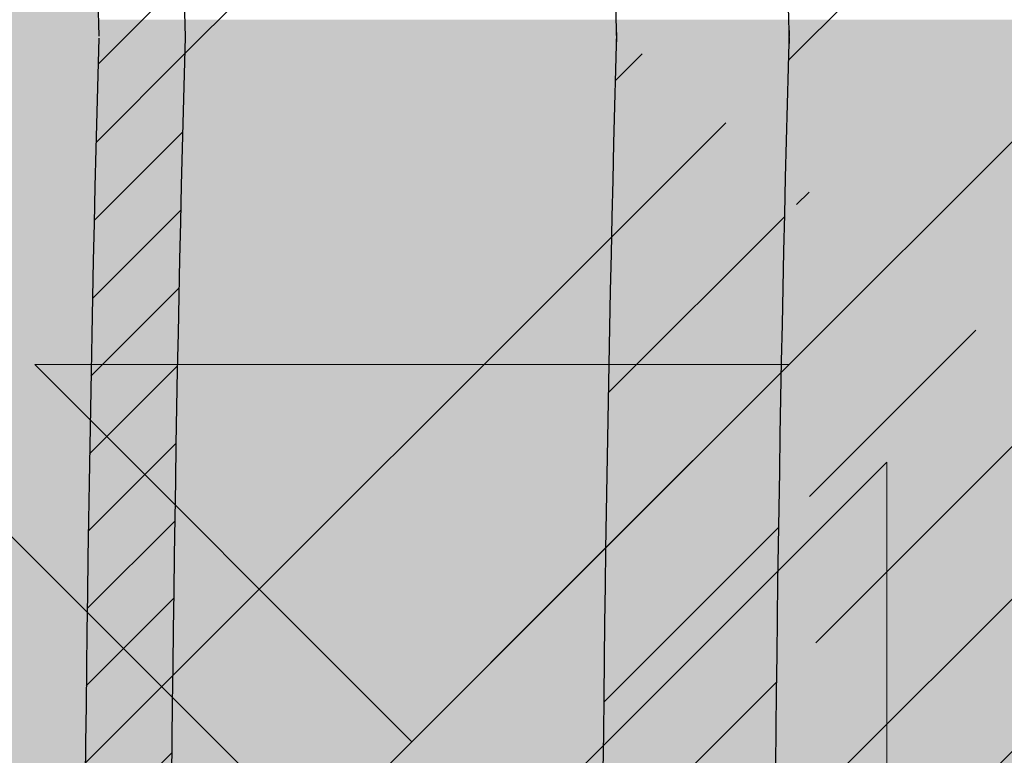
# Model space of a CAD drawing. Units: inches. Extents: x 844 to 2234, y 346 to 1084.
# Tile 11 of 93: x 1119.118 to 1120.937, y 694.861 to 696.22. Entities that reach past the tile are written whole.
import ezdxf

# ---------------------------------------------------------------- set-up
doc = ezdxf.new("R2010")
doc.units = ezdxf.units.IN
doc.header["$MEASUREMENT"] = 0
for name, color, linetype, lineweight in [('A-ANNO-DIMS', 2, 'Continuous', 18), ('furniture', 8, 'Continuous', 18), ('RA-AP-01$0$INT', 35, 'Continuous', 5)]:
    doc.layers.add(name, color=color, linetype=linetype, lineweight=lineweight)
doc.layers.add('RA-AP-01$0$FURN', color=3, linetype='Continuous')
doc.layers.add('RA-AP-01$0$WOOD', color=64, linetype='Continuous')
doc.styles.get("Standard").update_dxf_attribs({"font": 'arial.ttf'})
doc.dimstyles.get("Standard").update_dxf_attribs({"dimtxt": 6, "dimasz": 3, "dimexe": 0.18, "dimexo": 0.0625, "dimgap": 0.09, "dimtad": 0, "dimtih": 1, "dimtoh": 1, "dimdec": 1, "dimzin": 0, "dimdsep": 46, "dimlunit": 3, "dimtxsty": 'Standard', "dimblk": 'ARCHTICK', "dimcen": 0.09, "dimadec": 0, "dimazin": 0, "dimtfac": 1, "dimtdec": 1, "dimtofl": 0, "dimtmove": 0, "dimatfit": 3, "dimfxl": 1, "dimtolj": 1, "dimtzin": 0, "dimarcsym": 0})

# ---------------------------------------------------------------- blocks, each defined once
blk = doc.blocks.new('A$C18D01794')
at = {"layer": 'RA-AP-01$0$INT'}
h = blk.add_hatch(color=256, dxfattribs=at)
h.paths.add_polyline_path([(4.585917135068449, -6.356712009588271), (4.555206456959269, -6.35671200958746), (4.555206456959137, -6.387422687716308), (4.874495778835233, -6.706712009592356), (4.90520645695423, -6.676001331474049)])
h.paths.add_polyline_path([(5.255206456948813, -6.387422687716306), (5.255206456948682, -6.356712009605972), (5.224495778822613, -6.356712009605161), (4.905206456953498, -6.676001331474273), (4.935917135072151, -6.706712009592924)])
h.paths.add_polyline_path([(4.935917135072559, -6.706712009592068), (4.905206456953564, -6.737422687710376), (5.255206456951813, -7.087422687708613), (5.255206456951549, -7.026001331471008)])
h.paths.add_polyline_path([(4.555206456956399, -7.026001331471013), (4.555206456956134, -7.087422687708616), (4.905206456953821, -6.737422687710943), (4.874495778835166, -6.70671200959229)])
h = blk.add_hatch(color=256, dxfattribs=at)
h.paths.add_polyline_path([(4.585917135068448, -6.356712009588273), (4.614201406330596, -6.356712009589021), (4.668846067270487, -6.411356670531338), (4.723490728212344, -6.356712009591912), (4.771774999457151, -6.35671200959319), (4.826419660396886, -6.411356670535356), (4.862780050090322, -6.374996280843536), (4.844495778842715, -6.356712009595112), (4.862780050090411, -6.356712009595595), (4.905206456960182, -6.399138416468211), (4.947632863832445, -6.356712009597838), (4.965917135079675, -6.356712009598322), (4.947632863831759, -6.374996280845421), (4.983993253523576, -6.411356670538857), (5.038637914464627, -6.356712009600247), (5.08692218571208, -6.356712009601523), (5.141566846649976, -6.411356670541852), (5.196211507589851, -6.356712009604411), (5.224495778822615, -6.356712009605161), (4.905206456953975, -6.676001331473793)])
h.paths.add_polyline_path([(4.895206456956031, -6.637717060225675), (4.895206456958921, -6.528427738347902), (4.840561796018589, -6.583072399285802)], flags=16)
h.paths.add_polyline_path([(4.915206456955638, -6.637717060226121), (4.969851117895509, -6.583072399288678), (4.915206456957609, -6.528427738348344)], flags=16)
h.paths.add_polyline_path([(4.826419660395175, -6.568930263661755), (4.881064321335613, -6.514285602723745), (4.771774999456703, -6.514285602720857)], flags=16)
h.paths.add_polyline_path([(4.983993253519558, -6.568930263665262), (5.038637914460456, -6.514285602726792), (4.929348592581548, -6.514285602724816)], flags=16)
h.paths.add_polyline_path([(4.881064321336025, -6.494285602723742), (4.826419660397532, -6.439640941782821), (4.771774999457062, -6.494285602720859)], flags=16)
h.paths.add_polyline_path([(4.929348592582019, -6.494285602724817), (5.038637914460982, -6.494285602726792), (4.983993253522945, -6.439640941786327)], flags=16)
h.paths.add_polyline_path([(4.895206456960191, -6.480143467100443), (4.895206456962115, -6.407422687715913), (4.876922185715016, -6.389138416467584), (4.840561796021581, -6.425498806159401)], flags=16)
h.paths.add_polyline_path([(4.915206456958487, -6.480143467100889), (4.969851117899527, -6.425498806162279), (4.933490728206909, -6.389138416468043), (4.9152064569598, -6.40742268771434)], flags=16)
h.paths.add_polyline_path([(4.757632863832376, -6.480143467096812), (4.812277524772842, -6.425498806158772), (4.757632863834348, -6.370854145217844)], flags=16)
h.paths.add_polyline_path([(4.737632863832376, -6.480143467096286), (4.737632863834348, -6.370854145217375), (4.682988202893906, -6.425498806155385)], flags=16)
h.paths.add_polyline_path([(5.05278005008503, -6.480143467103376), (5.052780050087917, -6.370854145224413), (4.998135389146995, -6.425498806162908)], flags=16)
h.paths.add_polyline_path([(5.072780050085024, -6.480143467103744), (5.127424711025931, -6.42549880616527), (5.072780050087916, -6.370854145224832)], flags=16)
h.paths.add_polyline_path([(4.935917135072783, -6.706712009592292), (5.255206456948811, -6.387422687716309), (5.255206456948932, -6.415706958964177), (5.200561796010279, -6.470351619902839), (5.255206456949403, -6.524996280841948), (5.25520645694961, -6.5732805520894), (5.200561796009787, -6.627925213029239), (5.236922185702417, -6.664285602721864), (5.255206456949919, -6.646001331474357), (5.255206456949998, -6.664285602721898), (5.212780050078687, -6.706712009592262), (5.25520645695036, -6.749138416463932), (5.255206456950438, -6.767422687711313), (5.236922185702424, -6.749138416463297), (5.200561796009796, -6.785498806155928), (5.255206456950753, -6.840143467096874), (5.25520645695096, -6.888427738341682), (5.200561796010322, -6.943072399282328), (5.255206456951428, -6.997717060223427), (5.255206456951547, -7.026001331471006)])
h.paths.add_polyline_path([(5.042988202883395, -6.785498806155427), (5.097632863823085, -6.840143467095101), (5.097632863822622, -6.730854145216193)], flags=16)
h.paths.add_polyline_path([(5.028846067259663, -6.771356670531693), (5.083490728198774, -6.716712009592573), (4.974201406321001, -6.716712009593042)], flags=16)
h.paths.add_polyline_path([(5.117632863823087, -6.840143467095186), (5.172277524762331, -6.785498806155926), (5.11763286382262, -6.730854145216225)], flags=16)
h.paths.add_polyline_path([(5.08349072819877, -6.696712009593886), (5.028846067259652, -6.642067348654775), (4.974201406320998, -6.696712009593438)], flags=16)
h.paths.add_polyline_path([(5.131774999446817, -6.854285602718917), (5.186419660386065, -6.799640941779662), (5.241064321325782, -6.854285602719365)], flags=17)
h.paths.add_polyline_path([(5.131774999446228, -6.716712009592374), (5.186419660386065, -6.771356670532194), (5.222780050079488, -6.734996280838764), (5.204495778832781, -6.716712009592063)], flags=16)
h.paths.add_polyline_path([(5.097632863822613, -6.682569873970264), (5.097632863823061, -6.573280552091354), (5.042988202883383, -6.627925213031044)], flags=16)
h.paths.add_polyline_path([(5.131774999446899, -6.874285602718915), (5.241064321325809, -6.874285602719364), (5.186419660386591, -6.928930263658598)], flags=17)
h.paths.add_polyline_path([(5.131774999446226, -6.696712009594078), (5.204495778830767, -6.696712009594374), (5.22278005007868, -6.67842773834687), (5.186419660386049, -6.642067348654249)], flags=16)
h.paths.add_polyline_path([(5.11763286382262, -6.682569873970225), (5.17227752476232, -6.627925213030515), (5.117632863823064, -6.573280552091267)], flags=16)
h.paths.add_polyline_path([(5.186419660386069, -6.613783077405491), (5.241064321325754, -6.559138416465795), (5.131774999446791, -6.559138416466263)], flags=16)
h.paths.add_polyline_path([(5.131774999446872, -6.539138416466263), (5.24106432132578, -6.539138416465794), (5.186419660386554, -6.484493755526573)], flags=16)
h.paths.add_polyline_path([(5.255206456951811, -7.08742268770861), (5.255206456951895, -7.106712009588038), (4.555206456956052, -7.106712009588038), (4.555206456956136, -7.087422687708617), (4.905206456953973, -6.737422687710788)])
h.paths.add_polyline_path([(4.983993253513404, -6.8444937555241), (4.92934859257295, -6.899138416462108), (5.03863791445186, -6.899138416465014)], flags=16)
h.paths.add_polyline_path([(4.969851117889988, -6.83035161990006), (4.915206456952556, -6.775706958960171), (4.915206456949648, -6.884996280837944)], flags=16)
h.paths.add_polyline_path([(4.929348592572535, -6.919138416462105), (4.983993253511019, -6.973783077403037), (5.038637914451496, -6.919138416465012)], flags=16)
h.paths.add_polyline_path([(5.052780050074912, -6.93328055208906), (4.998135389134438, -6.987925213027088), (5.052780050072919, -7.042569873968025)], flags=16)
h.paths.add_polyline_path([(5.07278005007491, -6.933280552089588), (5.072780050072918, -7.042569873968497), (5.127424711013374, -6.987925213030498)], flags=16)
h.paths.add_polyline_path([(4.89520645695295, -6.775706958959721), (4.840561796013067, -6.830351619897157), (4.895206456950961, -6.884996280837494)], flags=16)
h.paths.add_polyline_path([(4.915206456948365, -6.933280552085403), (4.915206456946434, -7.006001331471951), (4.933490728192729, -7.024285602719066), (4.969851117886972, -6.987925213026453)], flags=16)
h.paths.add_polyline_path([(4.881064321327021, -6.899138416461022), (4.82641966038902, -6.84449375552057), (4.771774999448108, -6.899138416459029)], flags=16)
h.paths.add_polyline_path([(4.895206456950073, -6.933280552084951), (4.840561796009022, -6.987925213023558), (4.876922185700835, -7.024285602716997), (4.895206456948749, -7.006001331469487)], flags=16)
h.paths.add_polyline_path([(4.983993253510392, -7.0020673486505), (4.947632863816944, -7.038427738342319), (4.965917135064043, -7.05671200959023), (5.038637914448995, -7.056712009591555)], flags=16)
h.paths.add_polyline_path([(4.881064321326543, -6.91913841646102), (4.771774999447578, -6.919138416459031), (4.826419660385607, -6.973783077399508)], flags=16)
h.paths.add_polyline_path([(4.905206456946447, -7.014285602717636), (4.862780050074785, -7.056712009588352), (4.947632863816685, -7.056712009589775)], flags=16)
h.paths.add_polyline_path([(5.14156684663679, -7.002067348654549), (5.086922185696452, -7.056712009592438), (5.196211507574223, -7.056712009594425)], flags=16)
h.paths.add_polyline_path([(4.8264196603837, -7.002067348646972), (4.771774999442643, -7.056712009585575), (4.8444957788276, -7.056712009587508), (4.862780050075511, -7.038427738340416)], flags=16)
h.paths.add_polyline_path([(4.812277524760289, -6.98792521302292), (4.757632863822258, -6.933280552082447), (4.757632863819352, -7.042569873961408)], flags=16)
h.paths.add_polyline_path([(4.73763286382226, -6.933280552082079), (4.682988202881349, -6.987925213020536), (4.737632863819352, -7.04256987396099)], flags=16)
h.paths.add_polyline_path([(4.723490728195188, -7.056712009584289), (4.668846067257299, -7.002067348643949), (4.614201406317417, -7.056712009581383)], flags=16)
h.paths.add_polyline_path([(4.597632863829262, -6.706712009592262), (4.555206456957951, -6.664285602721896), (4.555206456958029, -6.646001331474357), (4.573490728205535, -6.664285602721864), (4.609851117898167, -6.627925213029238), (4.555206456958338, -6.573280552089402), (4.555206456958546, -6.524996280841952), (4.60985111789767, -6.470351619902839), (4.555206456959015, -6.415706958964177), (4.555206456959138, -6.387422687716309), (4.874495778835167, -6.70671200959229), (4.5552064569564, -7.026001331471015), (4.555206456956523, -6.997717060223433), (4.609851117897629, -6.94307239928233), (4.555206456956988, -6.888427738341681), (4.555206456957198, -6.840143467096881), (4.609851117898153, -6.78549880615593), (4.573490728205528, -6.749138416463297), (4.555206456957507, -6.76742268771132), (4.555206456957585, -6.749138416463933)])
h.paths.add_polyline_path([(4.712780050085332, -6.730854145216195), (4.712780050084863, -6.840143467095105), (4.767424711024555, -6.785498806155427)], flags=16)
h.paths.add_polyline_path([(4.726922185709173, -6.716712009592573), (4.781566846648288, -6.771356670531693), (4.836211507586949, -6.716712009593043)], flags=16)
h.paths.add_polyline_path([(4.692780050085327, -6.730854145216225), (4.638135389145619, -6.785498806155928), (4.692780050084865, -6.840143467095185)], flags=16)
h.paths.add_polyline_path([(4.726922185709182, -6.696712009593886), (4.836211507586949, -6.696712009593436), (4.7815668466483, -6.642067348654773)], flags=16)
h.paths.add_polyline_path([(4.678637914461726, -6.71671200959237), (4.605917135075169, -6.716712009592063), (4.587632863828464, -6.734996280838766), (4.623993253521887, -6.771356670532195)], flags=16)
h.paths.add_polyline_path([(4.712780050085336, -6.68256987397026), (4.767424711024568, -6.627925213031042), (4.71278005008489, -6.573280552091352)], flags=16)
h.paths.add_polyline_path([(4.678637914461726, -6.696712009594076), (4.623993253521899, -6.642067348654247), (4.587632863829271, -6.67842773834687), (4.605917135077185, -6.696712009594376)], flags=16)
h.paths.add_polyline_path([(4.692780050085336, -6.682569873970228), (4.692780050084889, -6.573280552091267), (4.638135389145632, -6.627925213030515)], flags=16)
h.paths.add_polyline_path([(4.623993253521885, -6.799640941779662), (4.678637914461131, -6.854285602718915), (4.56934859258217, -6.854285602719365)], flags=17)
h.paths.add_polyline_path([(4.623993253521901, -6.613783077405509), (4.678637914461158, -6.559138416466263), (4.569348592582195, -6.559138416465795)], flags=16)
h.paths.add_polyline_path([(4.678637914461051, -6.874285602718915), (4.623993253521361, -6.928930263658598), (4.569348592582143, -6.874285602719364)], flags=17)
h.paths.add_polyline_path([(4.678637914461076, -6.539138416466263), (4.623993253521399, -6.484493755526573), (4.569348592582167, -6.539138416465796)], flags=16)
h = blk.add_hatch(color=256, dxfattribs=at)
h.paths.add_polyline_path([(4.895206456952951, -6.77570695895972), (4.840561796013068, -6.830351619897156), (4.895206456950958, -6.884996280837495)])
h.paths.add_polyline_path([(4.915206456949649, -6.884996280837942), (4.969851117889987, -6.830351619900054), (4.915206456952556, -6.775706958960171)])
h.paths.add_polyline_path([(5.038637914451862, -6.899138416465013), (4.983993253513403, -6.8444937555241), (4.929348592572953, -6.899138416462106)])
h.paths.add_polyline_path([(4.929348592572535, -6.919138416462105), (4.983993253511018, -6.973783077403037), (5.038637914451497, -6.919138416465012)])
h.paths.add_polyline_path([(4.915206456948366, -6.933280552085397), (4.915206456946433, -7.006001331471951), (4.93349072819273, -7.024285602719068), (4.969851117886972, -6.987925213026454)])
h.paths.add_polyline_path([(5.038637914448995, -7.056712009591553), (4.983993253510389, -7.002067348650502), (4.947632863816946, -7.038427738342318), (4.965917135064043, -7.05671200959023)])
h.paths.add_polyline_path([(5.05278005007292, -7.042569873968023), (5.05278005007491, -6.933280552089059), (4.998135389134438, -6.987925213027088)])
h.paths.add_polyline_path([(5.07278005007292, -7.042569873968496), (5.127424711013374, -6.987925213030498), (5.072780050074909, -6.933280552089588)])
h.paths.add_polyline_path([(5.141566846636789, -7.002067348654547), (5.086922185696449, -7.056712009592438), (5.196211507574223, -7.056712009594425)])
h.paths.add_polyline_path([(4.947632863816688, -7.056712009589774), (4.905206456946449, -7.014285602717634), (4.862780050074784, -7.056712009588353)])
h.paths.add_polyline_path([(4.840561796009025, -6.987925213023556), (4.876922185700834, -7.024285602716997), (4.895206456948747, -7.006001331469488), (4.895206456950075, -6.933280552084953)])
h.paths.add_polyline_path([(4.88106432132654, -6.919138416461021), (4.771774999447577, -6.919138416459031), (4.826419660385606, -6.973783077399508)])
h.paths.add_polyline_path([(4.881064321327019, -6.899138416461022), (4.826419660389019, -6.844493755520571), (4.771774999448108, -6.89913841645903)])
h.paths.add_polyline_path([(4.757632863819352, -7.042569873961409), (4.812277524760284, -6.987925213022922), (4.757632863822259, -6.933280552082447)])
h.paths.add_polyline_path([(4.8264196603837, -7.002067348646974), (4.771774999442646, -7.056712009585575), (4.844495778827599, -7.05671200958751), (4.862780050075512, -7.038427738340417)])
h.paths.add_polyline_path([(4.737632863819352, -7.042569873960988), (4.737632863822258, -6.933280552082078), (4.682988202881349, -6.987925213020538)])
h.paths.add_polyline_path([(4.668846067257299, -7.002067348643952), (4.61420140631742, -7.056712009581384), (4.723490728195189, -7.056712009584292)])
for p, q in [((4.905206456953975, -6.737422687710788), (4.555206456956136, -7.087422687708617)), ((4.737632863822258, -6.933280552082079), (4.737632863819352, -7.042569873960989)), ((4.737632863819352, -7.042569873960989), (4.682988202881349, -6.987925213020538)), ((4.614201406317417, -7.056712009581383), (4.668846067257299, -7.002067348643951)), ((4.723490728195186, -7.056712009584289), (4.668846067257299, -7.002067348643951)), ((4.723490728195188, -7.056712009584293), (4.614201406317417, -7.056712009581383))]:
    blk.add_line(p, q, dxfattribs=at)
blk = doc.blocks.new('A$C32926AE1')
at = {"layer": 'RA-AP-01$0$FURN'}
h = blk.add_hatch(dxfattribs=at)
h.set_pattern_fill('ANSI31', color=256, scale=0.1, style=0)
h.set_pattern_definition([(45, (0, 0), (-0.0088388347648318, 0.0088388347648318), [])])
edge = h.paths.add_edge_path(flags=16)
edge.add_arc((4.904771284329206, 4.246793130718756), 0.2603971832811541, 75.22398030683196, 104.7760196931204)
edge.add_arc((4.904771284329206, 4.246793130718756), 0.2603971832811541, 75.223980306832, 104.77601969312039, ccw=False)
edge = h.paths.add_edge_path(flags=16)
edge.add_arc((4.904771284329206, 4.067062675376612), 0.2603971832811541, 255.2239803068796, 284.776019693168)
edge.add_arc((4.904771284329206, 4.067062675376612), 0.2603971832811541, 255.22398030687958, 284.77601969316805, ccw=False)
edge = h.paths.add_edge_path(flags=0)
edge.add_arc((4.904771284329206, 4.067062675376612), 0.2603971832811541, 255.2239803068796, 284.776019693168)
edge.add_arc((4.904771284329206, 4.067062675376612), 0.2603971832811541, 255.22398030687958, 284.77601969316805, ccw=False)
edge = h.paths.add_edge_path(flags=0)
edge.add_arc((4.904771284329206, 4.067062675376612), 0.2603971832811541, 255.2239803068796, 284.776019693168)
edge.add_arc((4.904771284329206, 4.067062675376612), 0.2603971832811541, 255.22398030687958, 284.77601969316805, ccw=False)
edge = h.paths.add_edge_path()
edge.add_arc((4.604388392048174, 4.588829985554312), 0.1599999999999918, 342.3781640246255, 354.4317409793762)
edge.add_arc((5.090145208887507, 4.43216705527679), 0.3503971832811637, 162.0091218307731, 180.3186872093483)
edge.add_arc((5.205154176610243, 4.588829985554953), 0.1599999999999917, 185.5682590208461, 197.6218359767349)
edge.add_arc((4.904771284329229, 4.246793130718735), 0.3503971832811761, 72.00912183053516, 107.9908781690354)
edge.add_arc((9.535952835716557, 4.28682295566602), 4.798342501046485, 178.2875002453811, 181.5576802719453)
edge.add_arc((4.719397359771122, 4.43216705527679), 0.3503971832811637, 359.6813127906516, 377.9908781692269)
edge.add_arc((9.535967292294904, 4.286822350292874), 4.778371420254705, 178.2965938931842, 181.5667745797229)
edge.add_arc((4.719397359771122, 4.43216705527679), 0.3303971832811637, 359.6813127906516, 377.9908781692269)
edge.add_arc((0.2735752763637294, 4.286822350292874), 4.7783714202547, 358.4332254202771, 361.7034061068158)
edge.add_arc((5.061434214606998, 4.732549947558029), 0.1600000000000254, 252.3781640250584, 264.4317409792362)
edge.add_arc((4.748108354051257, 4.732549947558012), 0.1600000000000541, 275.5682590208426, 287.6218359759532)
edge.add_arc((4.604388392048115, 4.588829985554317), 0.1800000000000505, 342.3567572500182, 349.3735009646207)
edge.add_arc((5.205154176610254, 4.588829985554976), 0.1800000000000069, 190.6264990356027, 197.6432427513933)
edge.add_arc((5.061434214607106, 4.732549947558013), 0.1800000000000424, 252.3567572496606, 259.3735009644582)
edge.add_arc((4.904771284329208, 4.246793130718737), 0.3303971832811676, 71.99844483668534, 108.0015551637021)
edge.add_arc((4.748108354051414, 4.732549947558045), 0.1800000000000547, 280.6264990355479, 287.6432427495938)
edge.add_arc((5.090145208887514, 4.432167055276789), 0.2803971832811691, 162.8706300666893, 180.816523289902)
edge.add_arc((4.719397359771136, 4.432167055276689), 0.2803971832811534, 359.183476710103, 377.1293699333214)
edge.add_arc((4.904771284329222, 4.246793130718737), 0.2803971832811769, 72.87063006672916, 107.1293699332334)
edge.add_arc((5.090145208887522, 4.432167055276788), 0.2603971832811776, 165.2239803068007, 180.9953123810312)
edge.add_arc((4.719397359771141, 4.432167055276699), 0.2603971832811458, 359.0046876189768, 374.7760196932087)
edge.add_arc((5.090145208887507, 4.43216705527679), 0.3303971832811637, 162.0091218307731, 180.3186872093483)
edge.add_arc((9.53595427642584, 4.285015535491528), 4.728345371032053, 178.265043920078, 181.5679956281801)
edge.add_arc((0.2735882922327999, 4.285015535491582), 4.728345371032045, 358.4320043718193, 361.7349560799204)
edge.add_arc((9.535953591267507, 4.284458026472751), 4.708343996644348, 178.2573054306777, 181.5704995759608)
edge.add_arc((0.273588977391114, 4.284458026472785), 4.708343996644358, 358.4295004240388, 361.7426945693213)
edge.add_arc((0.2735889773911131, 4.029397779622582), 4.708343996644359, 358.2573054306787, 361.5704995759613)
edge.add_arc((9.535953591267518, 4.029397779622618), 4.708343996644359, 178.4295004240391, 181.7426945693223)
edge.add_arc((0.2735882922327901, 4.028840270603786), 4.728345371032054, 358.2650439200796, 361.5679956281808)
edge.add_arc((9.53595427642584, 4.028840270603841), 4.728345371032054, 178.4320043718199, 181.7349560799219)
edge.add_arc((0.2735752763637302, 4.027033455802493), 4.778371420254699, 358.2965938931842, 361.5667745797229)
edge.add_arc((4.719397359771122, 3.881688750818578), 0.3303971832811637, 342.0091218307731, 360.3186872093484)
edge.add_arc((5.090145208887507, 3.881688750818578), 0.3303971832811637, 179.6813127906516, 197.9908781692269)
edge.add_arc((9.535967292294904, 4.027033455802493), 4.778371420254705, 178.433225420277, 181.7034061068158)
edge.add_arc((4.719397359771122, 3.881688750818578), 0.3503971832811637, 342.0091218307731, 360.3186872093484)
edge.add_arc((9.53595283571655, 4.027032850429349), 4.79834250104648, 178.4423197280546, 181.7124997546188)
edge.add_arc((4.719397359771141, 3.881688750818669), 0.2603971832811458, 345.2239803067913, 360.9953123810232)
edge.add_arc((5.090145208887522, 3.88168875081858), 0.2603971832811776, 179.0046876189687, 194.7760196931993)
edge.add_arc((4.904771284329222, 4.067062675376631), 0.2803971832811769, 252.8706300667665, 287.1293699332708)
edge.add_arc((4.719397359771136, 3.881688750818678), 0.2803971832811534, 342.8706300666787, 360.8165232898969)
edge.add_arc((5.090145208887514, 3.881688750818579), 0.2803971832811691, 179.183476710098, 197.1293699333106)
edge.add_arc((4.748108354051414, 3.581305858537323), 0.1800000000000547, 72.3567572504062, 79.37350096445199)
edge.add_arc((4.904771284329208, 4.067062675376631), 0.3303971832811676, 251.9984448362979, 288.0015551633146)
edge.add_arc((5.061434214607106, 3.581305858537355), 0.1800000000000424, 100.6264990355418, 107.6432427503394)
edge.add_arc((5.205154176610254, 3.725025820540392), 0.1800000000000069, 162.3567572486066, 169.3735009643972)
edge.add_arc((4.604388392048115, 3.725025820541051), 0.1800000000000505, 10.62649903537925, 17.64324274998182)
edge.add_arc((4.748108354051257, 3.581305858537356), 0.1600000000000541, 72.37816402404681, 84.43174097915735)
edge.add_arc((4.904771284329229, 4.067062675376632), 0.3503971832811761, 252.0091218309645, 287.9908781694648)
edge.add_arc((5.061434214606998, 3.581305858537339), 0.1600000000000254, 95.56825902076373, 107.6218359749416)
edge.add_arc((5.205154176610243, 3.725025820540414), 0.1599999999999917, 162.3781640232651, 174.4317409791539)
edge.add_arc((5.090145208887507, 3.881688750818578), 0.3503971832811637, 179.6813127906516, 197.9908781692269)
edge.add_arc((4.604388392048174, 3.725025820541056), 0.1599999999999918, 5.568259020623824, 17.62183597537444)
edge.add_arc((0.2735897329420762, 4.28682295566602), 4.798342501046482, 358.4423197280547, 361.7124997546188)
edge.add_arc((0.2735897329420691, 4.027032850429348), 4.798342501046489, 358.2875002453812, 361.5576802719453)
at = {"layer": 'RA-AP-01$0$WOOD'}
h = blk.add_hatch(color=256, dxfattribs=at)
h.dxf.hatch_style = 1
h.paths.add_polyline_path([(5.157430609644524, 4.573483066760929, -0.1009492694046607), (5.155401577623758, 4.593365984175333, -0.1842662638101597), (5.172249623284174, 4.638795604568598, 0.2056608120311276), (5.179560981299304, 4.661316324430096, 0.3614336704623542), (5.134352340494423, 4.706524965234944, 0.2056608120311297), (5.111831620632933, 4.699213607219793, -0.1842662638101113), (5.066402000239693, 4.682365561559342, -0.1055311479399994), (5.045656153913092, 4.68467289944697, 0.1567636581983829), (4.763886414745334, 4.684672899446966, -0.1055311479399895), (4.743140568418733, 4.68236556155934, -0.1842662638100833), (4.6977109480255, 4.69921360721979, 0.2056608120302612), (4.675190228164109, 4.706524965234949, 0.3614336704708441), (4.629981587358889, 4.66131632442871, 0.2056608120245944), (4.637292945374126, 4.638795604567974, -0.1842662638101024), (4.654140991034615, 4.59336598417475, -0.1009492694055169), (4.652111959013835, 4.573483066760181, 0.021410119221476), (4.629748025606143, 4.156712009541676, 0.0214101192214795), (4.652111959013809, 3.739940952323101, -0.1009492694059586), (4.654140991034615, 3.720058034908448, -0.1842662638100975), (4.637292945374126, 3.674628414515226, 0.2056608120245705), (4.629981587358889, 3.652107694654492, 0.3614336704708879), (4.675190228164113, 3.606899053848249, 0.2056608120302384), (4.697710948025501, 3.614210411863408, -0.1842662638100995), (4.743140568418738, 3.63105845752386, -0.1055311479402541), (4.763886414745388, 3.628751119636215, 0.1567636581983776), (5.045656153913137, 3.628751119636244, -0.1055311479397538), (5.066402000239692, 3.631058457523857, -0.1842662638101067), (5.111831620632931, 3.614210411863407, 0.2056608120310924), (5.134352340494417, 3.606899053848256, 0.3614336704624001), (5.179560981299307, 3.652107694653103, 0.2056608120311314), (5.172249623284175, 3.6746284145146, -0.1842662638101402), (5.155401577623758, 3.72005803490786, -0.1009492694051366), (5.15743060964455, 3.739940952322354, 0.0214101192215073), (5.179794543052287, 4.156712009541468, 0.0214101192215252)])
h.paths.add_polyline_path([(4.639748609479751, 4.156712009541513, 0.0213537860821624), (4.661970494867118, 3.741887061152232, -0.094075836301374), (4.664143710413708, 3.7196126951003, -0.1824818158568985), (4.644813765429836, 3.668037719127816, 0.2056608120245319), (4.639939526753007, 3.653023905887301, 0.3614336704710246), (4.676106439397173, 3.616856993242342, 0.2056608120302234), (4.691120252638095, 3.621731231919122, -0.1824818158602558), (4.742695228611606, 3.641061176902986, -0.1029891339458722), (4.766991894714349, 3.638256818950944, 0.156709409989566), (5.042550673941472, 3.638256818950105, -0.102989133958497), (5.066847340047078, 3.641061176902949, -0.1824818158594995), (5.118422316020358, 3.621731231919103, 0.2056608120311416), (5.133436129261316, 3.616856993242346, 0.3614336704621468), (5.169603041905217, 3.653023905886178, 0.2056608120310986), (5.164728803228477, 3.668037719127177, -0.1824818158565612), (5.145398858244737, 3.719612695099578, -0.0940758363009313), (5.147572073791232, 3.741887061151398, 0.0213537860822023), (5.169793959178681, 4.156712009541451, 0.0213537860822226), (5.147572073791203, 4.571536957931898, -0.0940758363005034), (5.145398858244737, 4.59381132398362, -0.1824818158565587), (5.164728803228476, 4.645386299956021, 0.2056608120311045), (5.169603041905216, 4.66040011319702, 0.3614336704621845), (5.133436129261313, 4.696567025840856, 0.2056608120310773), (5.118422316020359, 4.691692787164098, -0.182481815859508), (5.066847340047078, 4.67236284218025, -0.1029891339584606), (5.04255067394148, 4.675167200133092, 0.156709409989566), (4.766991894714357, 4.675167200132257, -0.1029891339458842), (4.742695228611611, 4.672362842180213, -0.1824818158602725), (4.691120252638095, 4.691692787164077, 0.2056608120302152), (4.676106439397174, 4.696567025840858, 0.3614336704710363), (4.639939526753005, 4.660400113195899, 0.2056608120245495), (4.644813765429837, 4.645386299955384, -0.1824818158568934), (4.664143710413708, 4.593811323982902, -0.0940758363009187), (4.661970494867149, 4.571536957931074, 0.021353786082177)], flags=16)
h.paths.add_polyline_path([(5.129794543052235, 4.432167055276933, -0.0141661062790638), (5.130152669293814, 4.156927903047693, -0.0141661062790647), (5.129794543052234, 3.881688750818433, -0.0785247771143638), (5.10979738006795, 3.755143611847103, 0.0945969212073497), (5.105408519571111, 3.717898134952927, 0.1043170707844957), (5.116074640131521, 3.670385395016088, 0.1043170707864965), (5.068561900193738, 3.681051515576561, 0.09459692119553), (5.031316423304057, 3.676662655080835, -0.1580239521427272), (4.778226145355827, 3.676662655080367, 0.0945969211986668), (4.740980668464973, 3.681051515576592, 0.1043170707882822), (4.693467928526415, 3.670385395015844, 0.1043170707867916), (4.704134049087309, 3.717898134953662, 0.0945969211972894), (4.69974518859162, 3.755143611844042, -0.0785247771163196), (4.679748025606343, 3.881688750818406, -0.0141661062790663), (4.679389899364763, 4.156927903047693, -0.0141661062790672), (4.679748025606343, 4.432167055276998, -0.0785247771163064), (4.699745188591625, 4.55871219425134, 0.094596921197333), (4.704134049087308, 4.595957671141738, 0.1043170707867205), (4.693467928526416, 4.643470411079523, 0.1043170707882628), (4.740980668464965, 4.632804290518776, 0.0945969211988114), (4.778226145355874, 4.637193151015016, -0.158023952142669), (5.031316423304015, 4.637193151014546, 0.0945969211956361), (5.068561900193736, 4.632804290518806, 0.1043170707864979), (5.11607464013152, 4.643470411079278, 0.1043170707844617), (5.105408519571112, 4.595957671142455, 0.0945969212074597), (5.109797380067959, 4.558712194248236, -0.0785247771143467)], flags=0)
h.paths.add_polyline_path([(5.119794532311105, 4.432259799204851, -0.0142000800617244), (5.120156169157484, 4.156927903047701, -0.0142000800617277), (5.119794532311105, 3.881596006890482, -0.0784894509520253), (5.100273383573699, 3.758192358677797, 0.0940138827242913), (5.095413455884425, 3.717477693979438, 0.0606271852308753), (5.099615656341024, 3.686844378806616, 0.0606271852322524), (5.068982341167493, 3.691046579263239, 0.0940138827010453), (5.028267676478798, 3.686186651576848, -0.1580706864508061), (4.781274892180912, 3.686186651576435, 0.0940138827026903), (4.740560227491556, 3.691046579263279, 0.0606271852339895), (4.709926912317155, 3.686844378806508, 0.0606271852329405), (4.714129112773991, 3.717477693980356, 0.094013882701304), (4.709269185087677, 3.758192358669163, -0.0784894509577193), (4.689748036347473, 3.881596006890469, -0.014200080061729), (4.689386399501094, 4.156927903047709, -0.0142000800617217), (4.689748036347473, 4.432259799204808, -0.078489450957724), (4.709269185087651, 4.555663447426125, 0.0940138827014585), (4.714129112773992, 4.596378112114996, 0.0606271852329731), (4.709926912317154, 4.62701142728886, 0.0606271852340196), (4.74056022749157, 4.622809226832087, 0.0940138827024997), (4.781274892180847, 4.627669154518912, -0.1580706864508359), (5.028267676478777, 4.627669154518526, 0.0940138827010946), (5.068982341167492, 4.622809226832129, 0.060627185232254), (5.099615656341024, 4.627011427288751, 0.0606271852308727), (5.095413455884425, 4.59637811211593, 0.0940138827241088), (5.100273383573675, 4.555663447417647, -0.0784894509520978)], flags=0)
h.paths.add_polyline_path([(5.06978912287499, 4.430218106756144, -0.014241683694547), (5.070173729147532, 4.156927903047672, -0.0142416836945458), (5.06978912287499, 3.883637699339223, -0.0800609523125196), (5.052662118612511, 3.773463122773442, 0.0526421978001116), (5.04590916754064, 3.740550867606997, 0.0526421977992423), (5.012996912374707, 3.73379791653534, -0.1583028414718258), (4.796545656286308, 3.73379791653451, 0.0526421978034211), (4.763633401117837, 3.740550867607021, 0.0526421978018622), (4.756880450045755, 3.773463122774558, -0.0800609523117106), (4.739753445783639, 3.883637699339268, -0.0142416836945435), (4.739368839511098, 4.156927903047671, -0.0142416836945477), (4.739753445783639, 4.430218106756155, -0.0800609523116345), (4.75688045004574, 4.540392683320762, 0.052642197801941), (4.763633401117837, 4.573304938488346, 0.0526421978035071), (4.796545656286361, 4.580057889560873, -0.1583028414717561), (5.012996912374669, 4.580057889560039, 0.0526421977993048), (5.04590916754064, 4.57330493848837, 0.0526421978002057), (5.052662118612529, 4.540392683321868, -0.080060952312477)], flags=0)
h.paths.add_polyline_path([(5.049789715110557, 4.43038092723357, -0.0143097550741839), (5.05018085590259, 4.156927903047715, -0.0143097550741854), (5.049789715110558, 3.883474878861827, -0.0800685599149176), (5.03362098255317, 3.779581877367999, 0.0306258898956367), (5.028241146483733, 3.758218888663947, 0.0306258898977031), (5.006878157778253, 3.75283905259408, -0.1583983521624096), (4.802664410878162, 3.752839052594731, 0.0306258898946014), (4.781301422174808, 3.758218888663924, 0.0306258898967912), (4.775921586105202, 3.779581877368794, -0.080068559914251), (4.759752853548071, 3.883474878861786, -0.0143097550741854), (4.759361712756037, 4.156927903047671, -0.0143097550741854), (4.759752853548071, 4.430380927233557, -0.0800685599142479), (4.775921586105193, 4.534273928726546, 0.0306258898968306), (4.781301422174808, 4.555636917431444, 0.0306258898945754), (4.802664410878143, 4.561016753500631, -0.1583983521624168), (5.006878157778244, 4.561016753501291, 0.0306258898977177), (5.028241146483733, 4.555636917431421, 0.0306258898958182), (5.03362098255321, 4.534273928727244, -0.080068559914796)], flags=0)
h.paths.add_polyline_path([(4.999766070382627, 4.428171244713864, -0.0143443147609634), (5.000198441819402, 4.156927903047689, -0.0143443147609612), (4.999766070382627, 3.885684561381556, -0.0784641635803329), (4.987356730658798, 3.799103304488872, -0.1506053783831347), (4.822185837999821, 3.79910330448882, -0.0784641635803318), (4.809776498276007, 3.885684561381509, -0.014344314760963), (4.809344126839227, 4.156927903047677, -0.0143443147609645), (4.809776498276007, 4.428171244713873, -0.0784641635803192), (4.822185837999822, 4.514752501606549, -0.1506053783831338), (4.987356730658798, 4.514752501606494, -0.078464163580285)], flags=0)
h.paths.add_polyline_path([(4.979755254238824, 4.42764379880488, -0.0143772539198268), (4.980205517789977, 4.156927903047693, -0.0143772539198275), (4.979755254238824, 3.886212007290489, -0.0689242507424422), (4.971183264704897, 3.815276770442801, -0.1296645318904179), (4.838359303953726, 3.815276770442746, -0.0689242507424186), (4.829787314419809, 3.886212007290419, -0.0143772539198292), (4.829337050868653, 4.156927903047653, -0.0143772539198325), (4.829787314419809, 4.427643798804946, -0.0689242507424211), (4.838359303953725, 4.498579035652621, -0.1296645318904187), (4.971183264704897, 4.498579035652565, -0.0689242507424401)], flags=0)
h = blk.add_hatch(color=256, dxfattribs=at)
h.dxf.hatch_style = 1
h.paths.add_polyline_path([(5.145398858244737, 4.59381132398362, -0.1824818158565616), (5.164728803228476, 4.645386299956021, 0.2056608120311045), (5.169603041905216, 4.66040011319702, 0.3614336704621845), (5.133436129261313, 4.696567025840856, 0.2056608120310773), (5.118422316020359, 4.691692787164098, -0.182481815859508), (5.066847340047078, 4.67236284218025, -0.1029891339584606), (5.04255067394148, 4.675167200133092, 0.156709409989566), (4.766991894714357, 4.675167200132257, -0.1029891339458842), (4.742695228611611, 4.672362842180213, -0.1824818158602725), (4.691120252638095, 4.691692787164077, 0.2056608120302152), (4.676106439397174, 4.696567025840858, 0.3614336704710363), (4.639939526753005, 4.660400113195899, 0.2056608120245495), (4.644813765429837, 4.645386299955384, -0.1824818158568934), (4.664143710413708, 4.593811323982902, -0.0940758363009187), (4.661970494867149, 4.571536957931074, 0.0213537860821772), (4.639748609479751, 4.156712009541507, 0.0213537860821625), (4.661970494867119, 3.741887061152226, -0.0940758363013071), (4.664143710413708, 3.719612695100309, -0.1824818158569294), (4.644813765429836, 3.668037719127816, 0.2056608120245319), (4.639939526753007, 3.653023905887301, 0.3614336704710246), (4.676106439397173, 3.616856993242342, 0.2056608120302234), (4.691120252638095, 3.621731231919122, -0.1824818158602558), (4.742695228611606, 3.641061176902986, -0.1029891339458722), (4.766991894714349, 3.638256818950944, 0.156709409989566), (5.042550673941472, 3.638256818950105, -0.102989133958497), (5.066847340047078, 3.641061176902949, -0.1824818158594995), (5.118422316020358, 3.621731231919103, 0.2056608120311416), (5.133436129261316, 3.616856993242346, 0.3614336704621468), (5.169603041905217, 3.653023905886178, 0.2056608120310986), (5.164728803228477, 3.668037719127177, -0.1824818158565612), (5.145398858244737, 3.719612695099578, -0.0940758363009313), (5.147572073791232, 3.741887061151398, 0.0213537860822023), (5.169793959178681, 4.156712009541451, 0.0213537860822226), (5.147572073791203, 4.571536957931898, -0.0940758363004996)])
h.paths.add_polyline_path([(5.109797380067958, 4.55871219424824, -0.0785247771143472), (5.129794543052234, 4.432167055276936, -0.0141661062790644), (5.130152669293814, 4.156927903047685, -0.014166106279066), (5.129794543052234, 3.881688750818401, -0.0785247771143517), (5.109797380067946, 3.755143611847092, 0.0945969212073132), (5.105408519571111, 3.717898134952929, 0.1043170707844995), (5.116074640131521, 3.670385395016088, 0.1043170707864965), (5.068561900193738, 3.681051515576561, 0.09459692119553), (5.031316423304057, 3.676662655080835, -0.1580239521427272), (4.778226145355827, 3.676662655080367, 0.0945969211986668), (4.740980668464973, 3.681051515576592, 0.1043170707882822), (4.693467928526415, 3.670385395015844, 0.1043170707867916), (4.704134049087309, 3.717898134953662, 0.0945969211972894), (4.69974518859162, 3.755143611844042, -0.0785247771163196), (4.679748025606343, 3.881688750818406, -0.0141661062790663), (4.679389899364763, 4.156927903047693, -0.0141661062790672), (4.679748025606343, 4.432167055276998, -0.0785247771163064), (4.699745188591625, 4.55871219425134, 0.094596921197333), (4.704134049087308, 4.595957671141738, 0.1043170707867205), (4.693467928526416, 4.643470411079523, 0.1043170707882628), (4.740980668464965, 4.632804290518776, 0.0945969211988114), (4.778226145355874, 4.637193151015016, -0.158023952142669), (5.031316423304015, 4.637193151014546, 0.0945969211956361), (5.068561900193736, 4.632804290518806, 0.1043170707864979), (5.11607464013152, 4.643470411079278, 0.1043170707844617), (5.105408519571112, 4.595957671142455, 0.0945969212074504)], flags=16)
h.paths.add_polyline_path([(5.100273383573655, 4.55566344741771, -0.0784894509521388), (5.119794532311105, 4.432259799204852, -0.0142000800617252), (5.120156169157484, 4.156927903047686, -0.014200080061726), (5.119794532311105, 3.881596006890502, -0.0784894509520446), (5.100273383573696, 3.758192358677786, 0.0940138827242721), (5.095413455884425, 3.717477693979436, 0.0606271852308692), (5.099615656341024, 3.686844378806616, 0.0606271852322522), (5.068982341167493, 3.691046579263239, 0.0940138827010453), (5.028267676478798, 3.686186651576848, -0.1580706864508061), (4.781274892180912, 3.686186651576435, 0.0940138827026903), (4.740560227491556, 3.691046579263279, 0.0606271852339895), (4.709926912317155, 3.686844378806508, 0.0606271852329405), (4.714129112773991, 3.717477693980356, 0.094013882701304), (4.709269185087677, 3.758192358669163, -0.0784894509577193), (4.689748036347473, 3.881596006890469, -0.014200080061729), (4.689386399501094, 4.156927903047709, -0.0142000800617217), (4.689748036347473, 4.432259799204808, -0.078489450957724), (4.709269185087651, 4.555663447426125, 0.0940138827014585), (4.714129112773992, 4.596378112114996, 0.0606271852329731), (4.709926912317154, 4.62701142728886, 0.0606271852340196), (4.74056022749157, 4.622809226832087, 0.0940138827024997), (4.781274892180847, 4.627669154518912, -0.1580706864508359), (5.028267676478777, 4.627669154518526, 0.0940138827010946), (5.068982341167492, 4.622809226832129, 0.060627185232254), (5.099615656341024, 4.627011427288751, 0.0606271852308727), (5.095413455884425, 4.59637811211593, 0.094013882723957)], flags=0)
h.paths.add_polyline_path([(5.04590916754064, 4.57330493848837, 0.0526421978002057), (5.052662118612529, 4.540392683321868, -0.0800609523124783), (5.06978912287499, 4.430218106756142, -0.0142416836945469), (5.070173729147532, 4.156927903047672, -0.0142416836945458), (5.06978912287499, 3.883637699339223, -0.0800609523125196), (5.052662118612511, 3.773463122773442, 0.0526421978001116), (5.04590916754064, 3.740550867606997, 0.0526421977992423), (5.012996912374707, 3.73379791653534, -0.1583028414718258), (4.796545656286308, 3.73379791653451, 0.0526421978034211), (4.763633401117837, 3.740550867607021, 0.0526421978018622), (4.756880450045755, 3.773463122774558, -0.0800609523117106), (4.739753445783639, 3.883637699339268, -0.0142416836945435), (4.739368839511098, 4.156927903047671, -0.0142416836945477), (4.739753445783639, 4.430218106756155, -0.0800609523116345), (4.75688045004574, 4.540392683320762, 0.052642197801941), (4.763633401117837, 4.573304938488346, 0.0526421978035071), (4.796545656286361, 4.580057889560873, -0.1583028414717561), (5.012996912374669, 4.580057889560039, 0.0526421977993048)], flags=0)
h.paths.add_polyline_path([(5.028241146483733, 4.555636917431422, 0.0306258898956949), (5.033620982553182, 4.534273928727329, -0.0800685599148649), (5.049789715110557, 4.430380927233569, -0.0143097550741839), (5.05018085590259, 4.156927903047715, -0.0143097550741854), (5.049789715110558, 3.883474878861827, -0.0800685599149176), (5.03362098255317, 3.779581877367999, 0.0306258898956367), (5.028241146483733, 3.758218888663947, 0.0306258898977031), (5.006878157778253, 3.75283905259408, -0.1583983521624096), (4.802664410878162, 3.752839052594731, 0.0306258898946014), (4.781301422174808, 3.758218888663924, 0.0306258898967912), (4.775921586105202, 3.779581877368794, -0.080068559914251), (4.759752853548071, 3.883474878861786, -0.0143097550741854), (4.759361712756037, 4.156927903047671, -0.0143097550741854), (4.759752853548071, 4.430380927233557, -0.0800685599142479), (4.775921586105193, 4.534273928726546, 0.0306258898968306), (4.781301422174808, 4.555636917431444, 0.0306258898945754), (4.802664410878143, 4.561016753500631, -0.1583983521624168), (5.006878157778244, 4.561016753501291, 0.0306258898977174)], flags=0)
h.paths.add_polyline_path([(4.987356730658798, 4.514752501606494, -0.0784641635803018), (4.999766070382627, 4.428171244713845, -0.0143443147609637), (5.000198441819402, 4.156927903047665, -0.0143443147609622), (4.999766070382628, 3.885684561381514, -0.0784641635802952), (4.987356730658797, 3.799103304488872, -0.1506053783831338), (4.822185837999821, 3.799103304488819, -0.0784641635803342), (4.809776498276007, 3.885684561381512, -0.0143443147609628), (4.809344126839227, 4.156927903047676, -0.0143443147609646), (4.809776498276007, 4.428171244713873, -0.0784641635803192), (4.822185837999822, 4.514752501606549, -0.1506053783831338)], flags=0)
h.paths.add_polyline_path([(4.971183264704897, 4.498579035652566, -0.0689242507424384), (4.979755254238824, 4.427643798804883, -0.0143772539198276), (4.980205517789977, 4.15692790304768, -0.0143772539198258), (4.979755254238823, 3.88621200729051, -0.0689242507424628), (4.971183264704897, 3.815276770442801, -0.129664531890417), (4.838359303953726, 3.815276770442746, -0.0689242507424186), (4.829787314419809, 3.886212007290419, -0.0143772539198292), (4.829337050868653, 4.156927903047653, -0.0143772539198325), (4.829787314419809, 4.427643798804946, -0.0689242507424211), (4.838359303953725, 4.498579035652621, -0.1296645318904187)], flags=0)
h = blk.add_hatch(dxfattribs=at)
h.set_pattern_fill('ANSI31', color=256, scale=0.05, style=0)
h.set_pattern_definition([(45, (0, 0), (-0.0044194173824159, 0.0044194173824159), [])])
h.paths.add_polyline_path([(5.130152669293814, 4.156927903047704, 0.0141661062790657), (5.129794543052234, 4.432167055276982, 0.0777827904001433), (5.110168979996553, 4.557559993161921, -0.0976515123401879), (5.105408519571111, 4.595957671142454, -0.1043170707844687), (5.116074640131522, 4.64347041107928), (5.099615656341024, 4.627011427288751, 0.0606271852308727), (5.095413455884425, 4.59637811211593, 0.0940138827241088), (5.100273383573675, 4.555663447417647, -0.0784894509520972), (5.119794532311105, 4.432259799204852, -0.0142000800617252), (5.120156169157484, 4.156927903047686, -0.014200080061726), (5.119794532311105, 3.881596006890502, -0.0784894509520446), (5.100273383573696, 3.758192358677786, 0.0940138827242721), (5.095413455884425, 3.717477693979436, 0.0606271852308692), (5.099615656341024, 3.686844378806616), (5.116074640131519, 3.67038539501609, -0.1043170707844594), (5.105408519571112, 3.717898134952912, -0.0976515123401594), (5.11016897999655, 3.756295812933435, 0.0777827904001654), (5.129794543052234, 3.881688750818409, 0.0141661062790665)])
h.paths.add_polyline_path([(5.030164222210597, 3.676291055149937, -0.0976515123472002), (5.068561900193739, 3.681051515576561, -0.1043170707864927), (5.116074640131521, 3.670385395016088), (5.099615656341024, 3.686844378806616, 0.0606271852322522), (5.068982341167493, 3.691046579263239, 0.0940138827010453), (5.028267676478798, 3.686186651576848, -0.1580706864508061), (4.781274892180912, 3.686186651576435, 0.0940138827026903), (4.740560227491556, 3.691046579263279, 0.0606271852339913), (4.709926912317154, 3.686844378806508), (4.693467928526416, 3.670385395015845, -0.1043170707882796), (4.740980668464973, 3.681051515576592, -0.0976515123427246), (4.779378346446416, 3.676291055150394, 0.156512506893803)])
h.paths.add_polyline_path([(4.689748036347473, 3.881596006890472, -0.014200080061729), (4.689386399501094, 4.156927903047712, -0.0142000800617195), (4.689748036347473, 4.432259799204768, -0.078489450957742), (4.709269185087648, 4.555663447426114, 0.0940138827014821), (4.714129112773992, 4.596378112114995, 0.0606271852329748), (4.709926912317154, 4.62701142728886), (4.693467928526414, 4.643470411079524, -0.1043170707867939), (4.704134049087309, 4.595957671141706, -0.09765151234893), (4.699373588660725, 4.557559993157876, 0.0777827903975372), (4.679748025606343, 4.432167055276987, 0.0141661062790675), (4.679389899364763, 4.156927903047675, 0.0141661062790641), (4.679748025606343, 3.88168875081843, 0.0777827903975637), (4.699373588660724, 3.756295812937497, -0.0976515123490278), (4.704134049087308, 3.717898134953629, -0.1043170707867196), (4.693467928526416, 3.670385395015845), (4.709926912317155, 3.686844378806508, 0.0606271852329413), (4.714129112773991, 3.717477693980357, 0.0940138827013084), (4.709269185087676, 3.758192358669166, -0.0784894509577192)])
h.paths.add_polyline_path([(4.779378346446434, 4.63756475094498, -0.0976515123427943), (4.740980668464964, 4.632804290518776, -0.1043170707882609), (4.693467928526416, 4.643470411079523), (4.709926912317154, 4.62701142728886, 0.0606271852340196), (4.74056022749157, 4.622809226832087, 0.0940138827024997), (4.781274892180847, 4.627669154518912, -0.1580706864508359), (5.028267676478777, 4.627669154518526, 0.0940138827010946), (5.068982341167492, 4.622809226832129, 0.060627185232254), (5.099615656341024, 4.627011427288751), (5.116074640131521, 4.643470411079279, -0.1043170707865022), (5.068561900193735, 4.632804290518806, -0.0976515123475899), (5.030164222210446, 4.637564750945479, 0.1565125068936924)])
h = blk.add_hatch(dxfattribs=at)
h.set_pattern_fill('ANSI32', color=256, scale=0.2, style=0)
h.set_pattern_definition([(45, (0, 0), (-0.0530330085889911, 0.0530330085889911), []), (45, (0.035355339, 0), (-0.0530330085889911, 0.0530330085889911), [])])
h.paths.add_polyline_path([(5.119794532311105, 4.432259799204823, 0.0777015974868765), (5.10065834347252, 4.554469821747928, -0.0968902511992216), (5.095413455884425, 4.596378112115931, -0.060627185230871), (5.099615656341024, 4.627011427288751, -0.060627185232254), (5.068982341167492, 4.622809226832129, -0.0968902512198245), (5.027074050790956, 4.628054114423209, 0.1564657949319105), (4.782468517866163, 4.628054114422785, -0.0968902512152247), (4.740560227491555, 4.622809226832088, -0.0606271852339878), (4.709926912317155, 4.627011427288859, -0.0606271852329413), (4.714129112773991, 4.596378112115011, -0.0968902512205338), (4.708884225182929, 4.554469821738175, 0.0777015974804443), (4.689748036347473, 4.43225979920482, 0.0142000800617215), (4.689386399501094, 4.156927903047726, 0.0142000800617273), (4.689748036347473, 3.88159600689052, 0.077701597480541), (4.708884225182985, 3.759385984357019, -0.096890251220082), (4.714129112773992, 3.717477693980371, -0.0606271852329731), (4.709926912317154, 3.686844378806507, -0.060627185233988), (4.740560227491554, 3.691046579263279, -0.0968902512152569), (4.782468517866175, 3.685801691672578, 0.1564657949319236), (5.027074050790988, 3.685801691672169, -0.0968902512197451), (5.068982341167491, 3.691046579263239, -0.0606271852322557), (5.099615656341024, 3.686844378806616, -0.0606271852308727), (5.095413455884425, 3.717477693979438, -0.0968902511991229), (5.100658343472507, 3.7593859843474, 0.0777015974868745), (5.119794532311105, 3.8815960068905, 0.014200080061726), (5.120156169157484, 4.156927903047685, 0.0142000800617238)])
h.paths.add_polyline_path([(5.070173729147531, 4.156927903047684, -0.0142416836945481), (5.06978912287499, 3.883637699339191, -0.0800609523125107), (5.052662118612505, 3.773463122773424, 0.0526421978000811), (5.04590916754064, 3.740550867606997, 0.0526421977993214), (5.012996912374658, 3.733797916535325, -0.1583028414717916), (4.796545656286304, 3.733797916534512, 0.0526421978034138), (4.763633401117837, 3.740550867607021, 0.0526421978018622), (4.756880450045755, 3.773463122774558, -0.0800609523117106), (4.739753445783639, 3.883637699339268, -0.0142416836945435), (4.739368839511098, 4.156927903047671, -0.0142416836945477), (4.739753445783639, 4.430218106756155, -0.0800609523116345), (4.75688045004574, 4.540392683320762, 0.052642197801941), (4.763633401117837, 4.573304938488346, 0.0526421978035071), (4.796545656286361, 4.580057889560873, -0.1583028414717561), (5.012996912374669, 4.580057889560039, 0.0526421977993048), (5.04590916754064, 4.57330493848837, 0.0526421978002057), (5.052662118612529, 4.540392683321868, -0.0800609523124783), (5.06978912287499, 4.430218106756142, -0.0142416836945463)], flags=16)
h.paths.add_polyline_path([(5.050180855902591, 4.156927903047686, -0.0143097550741856), (5.049789715110558, 3.883474878861795, -0.0800685599148126), (5.033620982553202, 3.7795818773681, 0.0306258898957837), (5.028241146483733, 3.758218888663947, 0.0306258898977031), (5.006878157778253, 3.75283905259408, -0.1583983521624096), (4.802664410878162, 3.752839052594731, 0.0306258898946014), (4.781301422174808, 3.758218888663924, 0.0306258898967912), (4.775921586105202, 3.779581877368794, -0.080068559914251), (4.759752853548071, 3.883474878861786, -0.0143097550741854), (4.759361712756037, 4.156927903047671, -0.0143097550741854), (4.759752853548071, 4.430380927233557, -0.0800685599142479), (4.775921586105193, 4.534273928726546, 0.0306258898968306), (4.781301422174808, 4.555636917431444, 0.0306258898945754), (4.802664410878143, 4.561016753500631, -0.1583983521624168), (5.006878157778244, 4.561016753501291, 0.0306258898977177), (5.028241146483733, 4.555636917431421, 0.0306258898958182), (5.03362098255321, 4.534273928727244, -0.0800685599147973), (5.049789715110557, 4.430380927233568, -0.0143097550741854)], flags=0)
h.paths.add_polyline_path([(5.000198441819402, 4.15692790304769, -0.0143443147609622), (4.999766070382627, 3.885684561381539, -0.0784641635803169), (4.987356730658798, 3.799103304488873, -0.1506053783831347), (4.822185837999821, 3.79910330448882, -0.0784641635803318), (4.809776498276007, 3.885684561381509, -0.014344314760963), (4.809344126839227, 4.156927903047677, -0.0143443147609645), (4.809776498276007, 4.428171244713873, -0.0784641635803192), (4.822185837999822, 4.514752501606549, -0.1506053783831338), (4.987356730658798, 4.514752501606494, -0.0784641635803018), (4.999766070382627, 4.428171244713845, -0.0143443147609624)], flags=0)
h.paths.add_polyline_path([(4.980205517789976, 4.156927903047707, -0.0143772539198295), (4.979755254238824, 3.886212007290466, -0.06892425074242), (4.971183264704897, 3.815276770442801, -0.129664531890417), (4.838359303953726, 3.815276770442746, -0.0689242507424186), (4.829787314419809, 3.886212007290419, -0.0143772539198292), (4.829337050868653, 4.156927903047653, -0.0143772539198325), (4.829787314419809, 4.427643798804946, -0.0689242507424211), (4.838359303953725, 4.498579035652621, -0.1296645318904187), (4.971183264704897, 4.498579035652565, -0.0689242507424418), (4.979755254238824, 4.427643798804878, -0.0143772539198259)], flags=0)
for centre, radius, start, end in [((9.535947846873398, 4.288228622620774), 4.858332530454219, 178.302242255809, 181.5473839997637), ((9.535954991989813, 4.288228324954387), 4.848346823659687, 178.3067023394723, 181.5518444050557), ((9.535952835716557, 4.28682295566602), 4.798342501046485, 178.2875002453811, 181.5576802719453), ((9.535967292294904, 4.286822350292874), 4.778371420254705, 178.2965938931842, 181.5667745797229), ((9.535947846873405, 4.025627183474595), 4.858332530454226, 178.4526160002362, 181.6977577441909), ((9.535954991989813, 4.025627481140981), 4.848346823659687, 178.4481555949443, 181.6932976605276), ((9.53595283571655, 4.027032850429349), 4.79834250104648, 178.4423197280546, 181.7124997546188), ((9.535967292294904, 4.027033455802493), 4.778371420254705, 178.433225420277, 181.7034061068158)]:
    blk.add_arc(centre, radius, start, end, dxfattribs=at)
blk = doc.blocks.new('A$C5D2F253E')
at = {"layer": 'RA-AP-01$0$FURN', "xscale": -0.7999999999883585, "yscale": 0.7999999999883585, "zscale": 0.8, "rotation": 90}
blk.add_blockref('A$C18D01794', (-5.687757199772477, 4.75791982714071), dxfattribs=at)
at = {"layer": 'RA-AP-01$0$WOOD', "rotation": 270}
blk.add_blockref('A$C32926AE1', (-4.161339601644158, 5.73852594588169), dxfattribs=at)
blk = doc.blocks.new('_ArchTick')
at = {"color": 0, "linetype": 'ByBlock', "const_width": 0.15}
blk.add_lwpolyline([(-0.5, -0.5), (0.5, 0.5)], dxfattribs=at)
blk = doc.blocks.new('*D144')
at = {"layer": 'A-ANNO-DIMS', "color": 0, "lineweight": -2, "transparency": 16777216}
for p, q in [((1096.615948, 439.3732739999999), (1096.615948, 1074.743301)), ((1143.115948, 492.373274), (1143.115948, 1074.743301)), ((1096.615948, 1074.563301), (1102.481950728513, 1074.563301)), ((1143.115948, 1074.563301), (1137.249945271487, 1074.563301))]:
    blk.add_line(p, q, dxfattribs=at)
at = {"layer": 'Defpoints', "color": 0, "transparency": 16777216}
for p in [(1143.115948, 1074.563301), (1143.115948, 492.3107739999999), (1096.615948, 439.3107739999999)]:
    blk.add_point(p, dxfattribs=at)
at = {"layer": 'A-ANNO-DIMS', "color": 0, "lineweight": -2, "transparency": 16777216, "xscale": 3, "yscale": 3, "zscale": 3, "rotation": 180}
blk.add_blockref('_ArchTick', (1096.615948, 1074.563301), dxfattribs=at)
at = {"layer": 'A-ANNO-DIMS', "color": 0, "lineweight": -2, "transparency": 16777216, "xscale": 3, "yscale": 3, "zscale": 3}
blk.add_blockref('_ArchTick', (1143.115948, 1074.563301), dxfattribs=at)
at = {"layer": 'A-ANNO-DIMS', "color": 0, "transparency": 16777216, "insert": (1119.865948, 1074.563301), "char_height": 6, "attachment_point": 5}
blk.add_mtext('\\A1;3\'-10 1/2"', dxfattribs=at)

msp = doc.modelspace()

# ---------------------------------------------------------------- block references
at = {"layer": 'furniture', "xscale": 15.94108302203742, "yscale": 15.94108302203742, "zscale": 15.94108302203742, "rotation": 90}
msp.add_blockref('A$C5D2F253E', (1136.147844094663, 696.2584716700112), dxfattribs=at)

# ---------------------------------------------------------------- dimensions: what is measured, and where the dimension line sits
at = {"layer": 'A-ANNO-DIMS'}
dim = msp.add_linear_dim(base=(1143.115948, 1074.563301), p1=(1096.615948, 439.3107739999999), p2=(1143.115948, 492.3107739999999), dimstyle='Standard', override={"dimdec": 1, "dimlfac": 1, "dimrnd": 0, "dimzin": 1, "dimdsep": 46, "dimlunit": 4, "dimfrac": 2}, dxfattribs=at)
dim.commit()
dim.dimension.update_dxf_attribs({"geometry": '*D144', "text_midpoint": (1119.865948, 1074.563301)})

doc.saveas('drawing.dxf')
